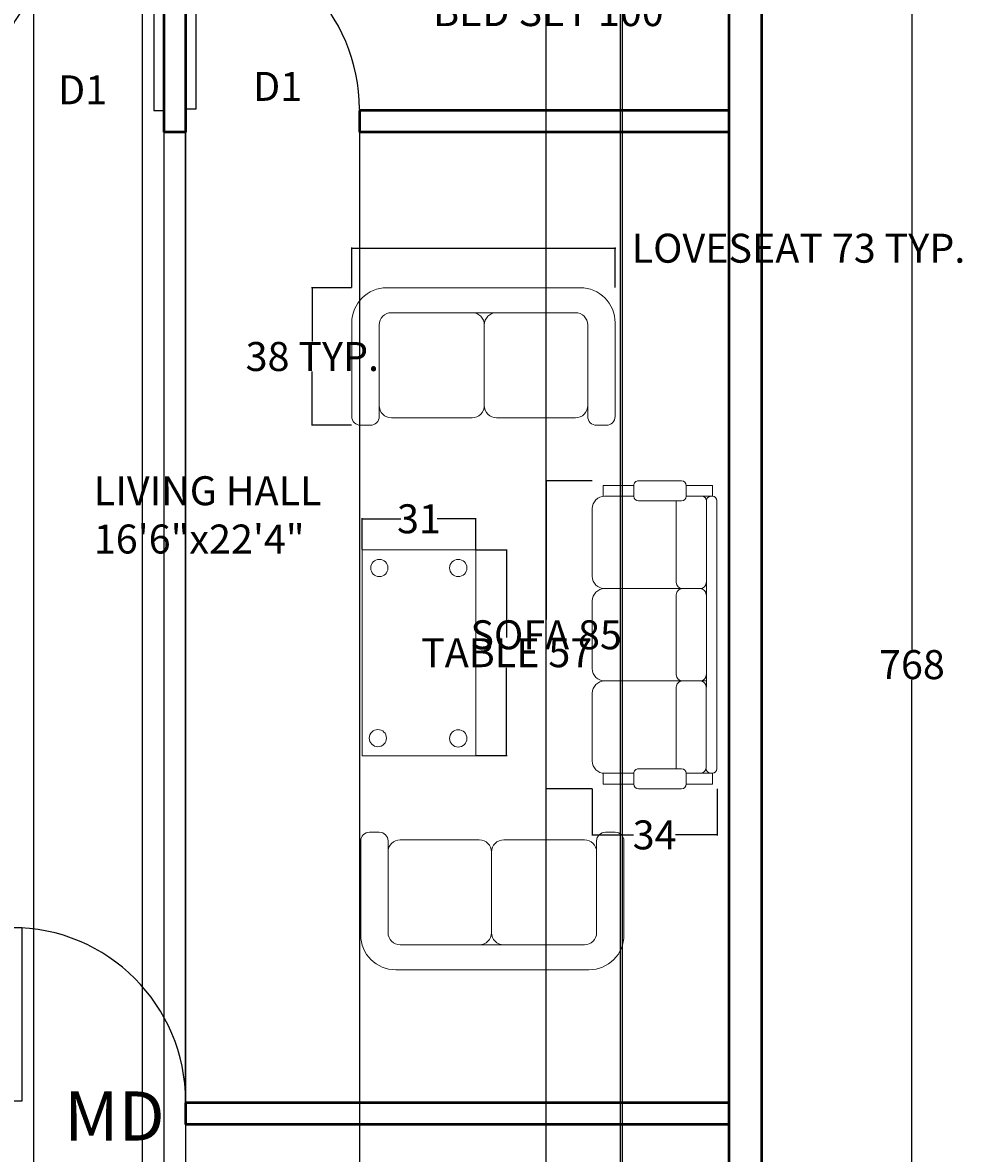
# Model space of a CAD drawing. Units: inches. Extents: x 3004 to 3478, y -798 to 114.
# Tile 4 of 5: x 3218 to 3478, y -503 to -190. Entities that reach past the tile are written whole.
import ezdxf

# ---------------------------------------------------------------- set-up
doc = ezdxf.new("R2010")
doc.units = ezdxf.units.IN
doc.header["$MEASUREMENT"] = 0
for name, color, linetype, lineweight in [('A-ANNO-DIMS', 2, 'Continuous', 18), ('A-ANNO-TEXT', 7, 'Continuous', 18), ('A-AREA-IDEN', 7, 'Continuous', 18), ('A-DOOR', 4, 'Continuous', 25), ('A-FURN', 8, 'Continuous', 18), ('A-WALL', 7, 'Continuous', 50)]:
    doc.layers.add(name, color=color, linetype=linetype, lineweight=lineweight)
doc.styles.get("Standard").update_dxf_attribs({"font": 'arial.ttf', "height": 8})
doc.dimstyles.get("Standard").update_dxf_attribs({"dimtxt": 0.18, "dimasz": 0.18, "dimexe": 0.18, "dimexo": 0.0625, "dimgap": 0.09, "dimtad": 0, "dimtih": 1, "dimtoh": 1, "dimzin": 0, "dimdsep": 46, "dimlunit": 4, "dimtxsty": 'Standard', "dimcen": 0.09, "dimadec": 0, "dimazin": 0, "dimtfac": 1, "dimtofl": 0, "dimtmove": 0, "dimatfit": 3, "dimfxl": 1, "dimtolj": 1, "dimtzin": 0, "dimarcsym": 0})

# ---------------------------------------------------------------- blocks, each defined once
blk = doc.blocks.new('F19')
for p, q in [((0.8306, 0.0191), (-0.9094, 0.0191)), ((-1.0094, -0.0109), (-0.9394, -0.0109)), ((-1.0094, -0.1809), (-1.0094, -0.0109)), ((-0.9394, -0.1809), (-0.9394, -0.0098)), ((-0.9394, -0.0109), (-0.9394, -0.0198)), ((0.213, -0.0498), (-0.9094, -0.0498)), ((-0.2985, -0.0498), (-0.387, -0.0498)), ((0.3015, -0.0498), (0.213, -0.0498)), ((0.2606, -0.6059), (0.2606, -0.0509)), ((0.3006, -0.0509), (0.8206, -0.0509)), ((0.9306, -0.0109), (0.8606, -0.0109)), ((0.8606, -0.0109), (0.8606, -0.0209)), ((0.8606, -0.0906), (0.8606, -0.0109)), ((0.9306, -0.1809), (0.9306, -0.0109)), ((-0.9394, -0.1773), (-0.9394, -0.0798)), ((-0.3394, -0.2054), (-0.3394, -0.0909)), ((0.2606, -0.2054), (0.2606, -0.0909)), ((0.8606, -0.1809), (0.8606, -0.0909)), ((-1.0394, -0.2109), (-1.0394, -0.4909)), ((-1.0094, -0.1809), (-0.9394, -0.1809)), ((-0.9094, -0.2109), (-0.9094, -0.4909)), ((-0.3394, -0.1546), (-0.3394, -0.6409)), ((0.2605, -0.3208), (0.2605, -0.174)), ((0.8306, -0.2109), (0.8306, -0.4909)), ((0.9306, -0.1809), (0.8606, -0.1809)), ((0.9606, -0.2109), (0.9606, -0.4909)), ((-0.3794, -0.2454), (-0.9114, -0.2454)), ((-0.3395, -0.3208), (-0.3395, -0.2854)), ((0.2206, -0.2454), (-0.2994, -0.2454)), ((0.2606, -0.2854), (0.2606, -0.6409)), ((0.829, -0.2454), (0.3006, -0.2454)), ((-1.0094, -0.5209), (-0.9394, -0.5209)), ((-1.0094, -0.7209), (-1.0094, -0.5209)), ((-0.9394, -0.5209), (-0.9394, -0.6909)), ((0.9306, -0.5209), (0.8606, -0.5209)), ((0.8606, -0.5209), (0.8606, -0.6909)), ((0.9306, -0.7209), (0.9306, -0.5209)), ((-0.9394, -0.6059), (-0.9394, -0.7109)), ((-0.9394, -0.6909), (-0.9394, -0.65)), ((-0.3394, -0.6059), (-0.3394, -0.7109)), ((0.2606, -0.6059), (0.2606, -0.7109)), ((0.8606, -0.6909), (0.8606, -0.65)), ((-0.9694, -0.7209), (-1.0094, -0.7209)), ((-0.9694, -0.7209), (-0.9393, -0.7209)), ((-0.9394, -0.6909), (-0.9394, -0.7109)), ((0.8906, -0.7209), (0.8605, -0.7209)), ((0.8606, -0.6909), (0.8606, -0.7109)), ((0.8906, -0.7209), (0.9306, -0.7209)), ((-0.4194, -0.7909), (-0.8594, -0.7909)), ((-0.4194, -0.7909), (-0.8594, -0.7909)), ((0.1806, -0.7909), (-0.2594, -0.7909)), ((0.0266, -0.7909), (0.0266, -0.7909)), ((0.7806, -0.7909), (0.3406, -0.7909))]:
    blk.add_line(p, q)
for centre, radius, start, end in [((-0.9094, -0.0109), 0.03, 90, 180), ((0.8306, -0.0109), 0.03, 360, 90), ((-0.9094, -0.0198), 0.03, 180, 270), ((-0.9094, -0.0798), 0.03, 90, 180), ((-0.3794, -0.0909), 0.04, 0, 90), ((-0.2994, -0.0909), 0.04, 90, 180), ((0.2206, -0.0909), 0.04, 0, 90), ((0.3006, -0.0909), 0.04, 90, 180), ((0.8206, -0.0909), 0.04, 0, 90), ((0.8306, -0.0209), 0.03, 270, 360), ((-1.0094, -0.2109), 0.03, 90, 180), ((-0.9394, -0.2109), 0.03, 0, 90), ((-0.3794, -0.2054), 0.04, 270, 360), ((-0.2994, -0.2054), 0.04, 180, 270), ((0.2206, -0.2054), 0.04, 270, 360), ((0.3006, -0.2054), 0.04, 180, 270), ((0.8606, -0.2109), 0.03, 90, 180), ((0.9306, -0.2109), 0.03, 0, 90), ((-1.0094, -0.4909), 0.03, 180, 270), ((-0.9394, -0.4909), 0.03, 270, 360), ((0.8606, -0.4909), 0.03, 180, 270), ((0.9306, -0.4909), 0.03, 270, 360), ((-0.8594, -0.7109), 0.08, 180, 270), ((-0.4194, -0.7109), 0.08, 270, 360), ((-0.4194, -0.7109), 0.08, 270, 360), ((-0.2594, -0.7109), 0.08, 180, 270), ((0.1806, -0.7109), 0.08, 270, 360), ((0.3406, -0.7109), 0.08, 180, 270), ((0.7806, -0.7109), 0.08, 270, 360)]:
    blk.add_arc(centre, radius, start, end)
blk = doc.blocks.new('A$C5C1B5EFD')
blk.add_blockref('F19', (1.0394, 0.7909))
blk = doc.blocks.new('A$C6BA70F2F')
for p, q in [((0.2, 0.7857), (1.3031, 0.7857)), ((0, 0.05), (0, 0.5857)), ((0.2263, 0.6431), (1.2768, 0.6431)), ((0.7563, 0.5835), (0.7563, 0.1071)), ((1.5031, 0.05), (1.5031, 0.5857)), ((0.1563, 0.05), (0.1563, 0.5731)), ((0.7563, 0.1131), (0.7563, 0.5731)), ((1.3468, 0.05), (1.3468, 0.5731)), ((0.6863, 0.0431), (0.2263, 0.0431)), ((1.2768, 0.0431), (0.8263, 0.0431)), ((0.1063, 0), (0.05, 0)), ((1.3968, 0), (1.4531, 0))]:
    blk.add_line(p, q)
for centre, radius, start, end in [((0.2, 0.5857), 0.2, 90, 180), ((1.3031, 0.5857), 0.2, 0, 90), ((0.2263, 0.5731), 0.07, 90, 180), ((0.6863, 0.5731), 0.07, 0, 90), ((0.8263, 0.5731), 0.07, 90, 180), ((1.2768, 0.5731), 0.07, 0, 90), ((0.2263, 0.1131), 0.07, 180, 270), ((0.6863, 0.1131), 0.07, 270, 0), ((0.8263, 0.1131), 0.07, 180, 270), ((1.2768, 0.1131), 0.07, 270, 0), ((0.05, 0.05), 0.05, 180, 270), ((0.1063, 0.05), 0.05, 270, 0), ((1.3968, 0.05), 0.05, 180, 270), ((1.4531, 0.05), 0.05, 270, 0)]:
    blk.add_arc(centre, radius, start, end)
blk = doc.blocks.new('table')
blk.add_lwpolyline([(-20.55, 0), (36.33, 0), (36.33, -31.34), (-20.55, -31.34)], close=True)
for centre in [(-15.51, -4.83), (31.56, -4.83), (-15.51, -26.62), (31.48, -27.03)]:
    blk.add_circle(centre, 2.38)
blk = doc.blocks.new('*U16')
for p, q in [((0, 0), (0, -100)), ((750, 0), (750, -100))]:
    blk.add_line(p, q)
blk.add_lwpolyline([(0, 0), (0, 750), (43.75, 750), (43.75, 0)], close=True)
blk.add_arc((0, 0), 750, 0, 90)
blk = doc.blocks.new('*U17')
for p, q in [((-750, 0), (-750, -100)), ((0, 0), (0, -100))]:
    blk.add_line(p, q)
blk.add_lwpolyline([(0, 0), (0, 750), (-43.75, 750), (-43.75, 0)], close=True)
blk.add_arc((0, 0), 750, 90, 180)
blk = doc.blocks.new('*D26')
at = {"layer": 'A-ANNO-DIMS', "color": 0, "lineweight": -2, "transparency": 16777216}
for p, q in [((3309.11, -263.53), (3309.11, -252.5)), ((3309.29, -252.68), (3381.63, -252.68)), ((3381.81, -263.53), (3381.81, -252.5)), ((3381.81, -252.68), (3381.99, -252.68))]:
    blk.add_line(p, q, dxfattribs=at)
at = {"layer": 'A-ANNO-DIMS', "color": 0, "transparency": 16777216}
for points in [[(3309.29, -252.65), (3309.29, -252.71), (3309.11, -252.68)], [(3381.63, -252.65), (3381.63, -252.71), (3381.81, -252.68)]]:
    blk.add_solid(points, dxfattribs=at)
at = {"layer": 'Defpoints', "color": 0, "transparency": 16777216}
for p in [(3381.81, -252.68), (3309.11, -263.59), (3381.81, -263.59)]:
    blk.add_point(p, dxfattribs=at)
at = {"layer": 'A-ANNO-DIMS', "color": 0, "transparency": 16777216, "insert": (3432.43, -252.68), "char_height": 8, "attachment_point": 5}
blk.add_mtext('\\A1;LOVESEAT 73 TYP.', dxfattribs=at)
blk = doc.blocks.new('*D27')
at = {"layer": 'A-ANNO-DIMS', "color": 0, "lineweight": -2, "transparency": 16777216}
for p, q in [((3309.04, -263.59), (3298.02, -263.59)), ((3298.2, -263.77), (3298.2, -278.41)), ((3298.2, -301.41), (3298.2, -286.77)), ((3309.04, -301.59), (3298.02, -301.59))]:
    blk.add_line(p, q, dxfattribs=at)
at = {"layer": 'A-ANNO-DIMS', "color": 0, "transparency": 16777216}
for points in [[(3298.17, -263.77), (3298.23, -263.77), (3298.2, -263.59)], [(3298.17, -301.41), (3298.23, -301.41), (3298.2, -301.59)]]:
    blk.add_solid(points, dxfattribs=at)
at = {"layer": 'Defpoints', "color": 0, "transparency": 16777216}
for p in [(3298.2, -263.59), (3309.11, -263.59), (3309.11, -301.59)]:
    blk.add_point(p, dxfattribs=at)
at = {"layer": 'A-ANNO-DIMS', "color": 0, "transparency": 16777216, "insert": (3298.2, -282.59), "char_height": 8, "attachment_point": 5}
blk.add_mtext('\\A1;38 TYP.', dxfattribs=at)
blk = doc.blocks.new('*D32')
at = {"layer": 'A-ANNO-DIMS', "color": 0, "lineweight": -2, "transparency": 16777216}
for p, q in [((3375.44, -316.93), (3362.58, -316.93)), ((3362.76, -317.11), (3362.76, -355.21)), ((3362.76, -401.77), (3362.76, -363.67)), ((3375.44, -401.95), (3362.58, -401.95))]:
    blk.add_line(p, q, dxfattribs=at)
at = {"layer": 'A-ANNO-DIMS', "color": 0, "transparency": 16777216}
for points in [[(3362.73, -317.11), (3362.79, -317.11), (3362.76, -316.93)], [(3362.73, -401.77), (3362.79, -401.77), (3362.76, -401.95)]]:
    blk.add_solid(points, dxfattribs=at)
at = {"layer": 'Defpoints', "color": 0, "transparency": 16777216}
for p in [(3375.51, -316.93), (3362.76, -401.95), (3375.51, -401.95)]:
    blk.add_point(p, dxfattribs=at)
at = {"layer": 'A-ANNO-DIMS', "color": 0, "transparency": 16777216, "insert": (3362.76, -359.44), "char_height": 8, "attachment_point": 5}
blk.add_mtext('\\A1;SOFA 85', dxfattribs=at)
blk = doc.blocks.new('*D33')
at = {"layer": 'A-ANNO-DIMS', "color": 0, "lineweight": -2, "transparency": 16777216}
for p, q in [((3375.51, -402.01), (3375.51, -414.88)), ((3409.94, -402.01), (3409.94, -414.88)), ((3375.69, -414.7), (3386.92, -414.7)), ((3409.76, -414.7), (3398.52, -414.7))]:
    blk.add_line(p, q, dxfattribs=at)
at = {"layer": 'A-ANNO-DIMS', "color": 0, "transparency": 16777216}
for points in [[(3375.69, -414.67), (3375.69, -414.73), (3375.51, -414.7)], [(3409.76, -414.67), (3409.76, -414.73), (3409.94, -414.7)]]:
    blk.add_solid(points, dxfattribs=at)
at = {"layer": 'Defpoints', "color": 0, "transparency": 16777216}
for p in [(3375.51, -401.95), (3409.94, -401.95), (3409.94, -414.7)]:
    blk.add_point(p, dxfattribs=at)
at = {"layer": 'A-ANNO-DIMS', "color": 0, "transparency": 16777216, "insert": (3392.72, -414.7), "char_height": 8, "attachment_point": 5}
blk.add_mtext('\\A1;34', dxfattribs=at)
blk = doc.blocks.new('*D34')
at = {"layer": 'A-ANNO-DIMS', "color": 0, "lineweight": -2, "transparency": 16777216}
for p, q in [((3313.57, -172.46), (3313.57, -187.52)), ((3413.21, -172.46), (3413.21, -187.52)), ((3313.75, -187.34), (3329.19, -187.34)), ((3413.03, -187.34), (3397.59, -187.34))]:
    blk.add_line(p, q, dxfattribs=at)
at = {"layer": 'A-ANNO-DIMS', "color": 0, "transparency": 16777216}
for points in [[(3313.75, -187.31), (3313.75, -187.37), (3313.57, -187.34)], [(3413.03, -187.31), (3413.03, -187.37), (3413.21, -187.34)]]:
    blk.add_solid(points, dxfattribs=at)
at = {"layer": 'Defpoints', "color": 0, "transparency": 16777216}
for p in [(3313.57, -172.39), (3413.21, -172.39), (3413.21, -187.34)]:
    blk.add_point(p, dxfattribs=at)
at = {"layer": 'A-ANNO-DIMS', "color": 0, "transparency": 16777216, "insert": (3363.39, -187.34), "char_height": 8, "attachment_point": 5}
blk.add_mtext('\\A1;BED SET 100', dxfattribs=at)
blk = doc.blocks.new('*D36')
at = {"layer": 'A-ANNO-DIMS', "color": 0, "lineweight": -2, "transparency": 16777216}
for p, q in [((3343.39, -335.95), (3352.04, -335.95)), ((3351.86, -336.13), (3351.86, -360.23)), ((3351.86, -392.64), (3351.86, -368.54)), ((3343.39, -392.82), (3352.04, -392.82))]:
    blk.add_line(p, q, dxfattribs=at)
at = {"layer": 'A-ANNO-DIMS', "color": 0, "transparency": 16777216}
for points in [[(3351.83, -336.13), (3351.89, -336.13), (3351.86, -335.95)], [(3351.83, -392.64), (3351.89, -392.64), (3351.86, -392.82)]]:
    blk.add_solid(points, dxfattribs=at)
at = {"layer": 'Defpoints', "color": 0, "transparency": 16777216}
for p in [(3343.33, -335.95), (3343.33, -392.82), (3351.86, -392.82)]:
    blk.add_point(p, dxfattribs=at)
at = {"layer": 'A-ANNO-DIMS', "color": 0, "transparency": 16777216, "insert": (3351.86, -364.39), "char_height": 8, "attachment_point": 5}
blk.add_mtext('\\A1;TABLE 57', dxfattribs=at)
blk = doc.blocks.new('*D37')
at = {"layer": 'A-ANNO-DIMS', "color": 0, "lineweight": -2, "transparency": 16777216}
for p, q in [((3311.98, -335.88), (3311.98, -327.23)), ((3312.16, -327.41), (3322.61, -327.41)), ((3343.15, -327.41), (3332.7, -327.41)), ((3343.33, -335.88), (3343.33, -327.23))]:
    blk.add_line(p, q, dxfattribs=at)
at = {"layer": 'A-ANNO-DIMS', "color": 0, "transparency": 16777216}
for points in [[(3312.16, -327.38), (3312.16, -327.44), (3311.98, -327.41)], [(3343.15, -327.38), (3343.15, -327.44), (3343.33, -327.41)]]:
    blk.add_solid(points, dxfattribs=at)
at = {"layer": 'Defpoints', "color": 0, "transparency": 16777216}
for p in [(3343.33, -327.41), (3311.98, -335.95), (3343.33, -335.95)]:
    blk.add_point(p, dxfattribs=at)
at = {"layer": 'A-ANNO-DIMS', "color": 0, "transparency": 16777216, "insert": (3327.65, -327.41), "char_height": 8, "attachment_point": 5}
blk.add_mtext('\\A1;31', dxfattribs=at)
blk = doc.blocks.new('*D39')
at = {"layer": 'A-ANNO-DIMS', "color": 0, "lineweight": -2, "transparency": 16777216}
for p, q in [((3422.27, 16.32), (3463.94, 16.32)), ((3463.76, 16.14), (3463.76, -363.5)), ((3463.76, -751.5), (3463.76, -371.85)), ((3422.27, -751.68), (3463.94, -751.68))]:
    blk.add_line(p, q, dxfattribs=at)
at = {"layer": 'A-ANNO-DIMS', "color": 0, "transparency": 16777216}
for points in [[(3463.73, 16.14), (3463.79, 16.14), (3463.76, 16.32)], [(3463.73, -751.5), (3463.79, -751.5), (3463.76, -751.68)]]:
    blk.add_solid(points, dxfattribs=at)
at = {"layer": 'Defpoints', "color": 0, "transparency": 16777216}
for p in [(3422.21, 16.32), (3422.21, -751.68), (3463.76, -751.68)]:
    blk.add_point(p, dxfattribs=at)
at = {"layer": 'A-ANNO-DIMS', "color": 0, "transparency": 16777216, "insert": (3463.76, -367.68), "char_height": 8, "attachment_point": 5}
blk.add_mtext('\\A1;768', dxfattribs=at)
blk = doc.blocks.new('*D44')
at = {"layer": 'A-ANNO-DIMS', "color": 0, "lineweight": -2, "transparency": 16777216}
for p, q in [((3257.211316, -220.74039), (3257.211316, -793.40789)), ((3263.211316, -220.74039), (3263.211316, -793.40789)), ((3257.031316, -793.22789), (3256.851316, -793.22789)), ((3263.391316, -793.22789), (3263.571316, -793.22789))]:
    blk.add_line(p, q, dxfattribs=at)
at = {"layer": 'A-ANNO-DIMS', "color": 0, "transparency": 16777216}
for points in [[(3257.031316, -793.19789), (3257.031316, -793.25789), (3257.211316, -793.22789)], [(3263.391316, -793.19789), (3263.391316, -793.25789), (3263.211316, -793.22789)]]:
    blk.add_solid(points, dxfattribs=at)
at = {"layer": 'Defpoints', "color": 0, "transparency": 16777216}
for p in [(3257.211316, -220.67789), (3263.211316, -220.67789), (3263.211316, -793.22789)]:
    blk.add_point(p, dxfattribs=at)
at = {"layer": 'A-ANNO-DIMS', "color": 0, "transparency": 16777216, "insert": (3260.211316, -793.22789), "char_height": 8, "attachment_point": 5}
blk.add_mtext('\\A1;6', dxfattribs=at)
blk = doc.blocks.new('*D45')
at = {"layer": 'A-ANNO-DIMS', "color": 0, "lineweight": -2, "transparency": 16777216}
for p, q in [((3422.21, 16.26), (3422.21, -793.41)), ((3413.21, 7.26), (3413.21, -793.41)), ((3413.39, -793.23), (3414.99, -793.23)), ((3422.03, -793.23), (3420.43, -793.23))]:
    blk.add_line(p, q, dxfattribs=at)
at = {"layer": 'A-ANNO-DIMS', "color": 0, "transparency": 16777216}
for points in [[(3413.39, -793.2), (3413.39, -793.26), (3413.21, -793.23)], [(3422.03, -793.2), (3422.03, -793.26), (3422.21, -793.23)]]:
    blk.add_solid(points, dxfattribs=at)
at = {"layer": 'Defpoints', "color": 0, "transparency": 16777216}
for p in [(3422.21, 16.32), (3413.21, 7.32), (3422.21, -793.23)]:
    blk.add_point(p, dxfattribs=at)
at = {"layer": 'A-ANNO-DIMS', "color": 0, "transparency": 16777216, "insert": (3417.71, -793.23), "char_height": 8, "attachment_point": 5}
blk.add_mtext('\\A1;9', dxfattribs=at)
blk = doc.blocks.new('*D46')
at = {"layer": 'A-ANNO-DIMS', "color": 0, "lineweight": -2, "transparency": 16777216}
for p, q in [((3263.21, -214.34), (3263.21, -793.41)), ((3311.21, -214.74), (3311.21, -793.41)), ((3263.39, -793.23), (3281.22, -793.23)), ((3311.03, -793.23), (3293.2, -793.23))]:
    blk.add_line(p, q, dxfattribs=at)
at = {"layer": 'A-ANNO-DIMS', "color": 0, "transparency": 16777216}
for points in [[(3263.39, -793.2), (3263.39, -793.26), (3263.21, -793.23)], [(3311.03, -793.2), (3311.03, -793.26), (3311.21, -793.23)]]:
    blk.add_solid(points, dxfattribs=at)
at = {"layer": 'Defpoints', "color": 0, "transparency": 16777216}
for p in [(3263.21, -214.28), (3311.21, -214.68), (3311.21, -793.23)]:
    blk.add_point(p, dxfattribs=at)
at = {"layer": 'A-ANNO-DIMS', "color": 0, "transparency": 16777216, "insert": (3287.21, -793.23), "char_height": 8, "attachment_point": 5}
blk.add_mtext('\\A1;48', dxfattribs=at)
blk = doc.blocks.new('*D47')
at = {"layer": 'A-ANNO-DIMS', "color": 0, "lineweight": -2, "transparency": 16777216}
for p, q in [((3413.21, -42.74), (3413.21, -793.41)), ((3383.21, -46.74), (3383.21, -793.41)), ((3383.39, -793.23), (3392.41, -793.23)), ((3413.03, -793.23), (3404.01, -793.23))]:
    blk.add_line(p, q, dxfattribs=at)
at = {"layer": 'A-ANNO-DIMS', "color": 0, "transparency": 16777216}
for points in [[(3383.39, -793.2), (3383.39, -793.26), (3383.21, -793.23)], [(3413.03, -793.2), (3413.03, -793.26), (3413.21, -793.23)]]:
    blk.add_solid(points, dxfattribs=at)
at = {"layer": 'Defpoints', "color": 0, "transparency": 16777216}
for p in [(3413.21, -42.68), (3383.21, -46.68), (3413.21, -793.23)]:
    blk.add_point(p, dxfattribs=at)
at = {"layer": 'A-ANNO-DIMS', "color": 0, "transparency": 16777216, "insert": (3398.21, -793.23), "char_height": 8, "attachment_point": 5}
blk.add_mtext('\\A1;30', dxfattribs=at)
blk = doc.blocks.new('*D55')
at = {"layer": 'A-ANNO-DIMS', "color": 0, "lineweight": -2, "transparency": 16777216}
for p, q in [((3215.21, -494.62), (3215.21, 109.05)), ((3215.39, 108.87), (3233.22, 108.87)), ((3263.03, 108.87), (3245.2, 108.87)), ((3263.21, -494.62), (3263.21, 109.05))]:
    blk.add_line(p, q, dxfattribs=at)
at = {"layer": 'A-ANNO-DIMS', "color": 0, "transparency": 16777216}
for points in [[(3215.39, 108.9), (3215.39, 108.84), (3215.21, 108.87)], [(3263.03, 108.9), (3263.03, 108.84), (3263.21, 108.87)]]:
    blk.add_solid(points, dxfattribs=at)
at = {"layer": 'Defpoints', "color": 0, "transparency": 16777216}
for p in [(3263.21, 108.87), (3215.21, -494.68), (3263.21, -494.68)]:
    blk.add_point(p, dxfattribs=at)
at = {"layer": 'A-ANNO-DIMS', "color": 0, "transparency": 16777216, "insert": (3239.21, 108.87), "char_height": 8, "attachment_point": 5}
blk.add_mtext('\\A1;48', dxfattribs=at)
blk = doc.blocks.new('*D59')
at = {"layer": 'A-ANNO-DIMS', "color": 0, "lineweight": -2, "transparency": 16777216}
for p, q in [((3362.72, -0.74), (3362.72, -793.41)), ((3383.72, -0.74), (3383.72, -793.41)), ((3362.9, -793.23), (3368.1, -793.23)), ((3383.54, -793.23), (3378.33, -793.23))]:
    blk.add_line(p, q, dxfattribs=at)
at = {"layer": 'A-ANNO-DIMS', "color": 0, "transparency": 16777216}
for points in [[(3362.9, -793.2), (3362.9, -793.26), (3362.72, -793.23)], [(3383.54, -793.2), (3383.54, -793.26), (3383.72, -793.23)]]:
    blk.add_solid(points, dxfattribs=at)
at = {"layer": 'Defpoints', "color": 0, "transparency": 16777216}
for p in [(3362.72, -0.68), (3383.72, -0.68), (3383.72, -793.23)]:
    blk.add_point(p, dxfattribs=at)
at = {"layer": 'A-ANNO-DIMS', "color": 0, "transparency": 16777216, "insert": (3373.22, -793.23), "char_height": 8, "attachment_point": 5}
blk.add_mtext('\\A1;21', dxfattribs=at)
blk = doc.blocks.new('*D63')
at = {"layer": 'A-ANNO-DIMS', "color": 0, "lineweight": -2, "transparency": 16777216}
for p, q in [((3221.21, -46.74), (3221.21, -793.41)), ((3251.21, -46.74), (3251.21, -793.41)), ((3221.39, -793.23), (3230.41, -793.23)), ((3251.03, -793.23), (3242.01, -793.23))]:
    blk.add_line(p, q, dxfattribs=at)
at = {"layer": 'A-ANNO-DIMS', "color": 0, "transparency": 16777216}
for points in [[(3221.39, -793.2), (3221.39, -793.26), (3221.21, -793.23)], [(3251.03, -793.2), (3251.03, -793.26), (3251.21, -793.23)]]:
    blk.add_solid(points, dxfattribs=at)
at = {"layer": 'Defpoints', "color": 0, "transparency": 16777216}
for p in [(3221.21, -46.68), (3251.21, -46.68), (3251.21, -793.23)]:
    blk.add_point(p, dxfattribs=at)
at = {"layer": 'A-ANNO-DIMS', "color": 0, "transparency": 16777216, "insert": (3236.21, -793.23), "char_height": 8, "attachment_point": 5}
blk.add_mtext('\\A1;30', dxfattribs=at)
blk = doc.blocks.new('*D64')
at = {"layer": 'A-ANNO-DIMS', "color": 0, "lineweight": -2, "transparency": 16777216}
for p, q in [((3215.21, -190.74), (3215.21, -793.41)), ((3257.21, -220.74), (3257.21, -793.41)), ((3215.39, -793.23), (3230.27, -793.23)), ((3257.03, -793.23), (3242.15, -793.23))]:
    blk.add_line(p, q, dxfattribs=at)
at = {"layer": 'A-ANNO-DIMS', "color": 0, "transparency": 16777216}
for points in [[(3215.39, -793.2), (3215.39, -793.26), (3215.21, -793.23)], [(3257.03, -793.2), (3257.03, -793.26), (3257.21, -793.23)]]:
    blk.add_solid(points, dxfattribs=at)
at = {"layer": 'Defpoints', "color": 0, "transparency": 16777216}
for p in [(3215.21, -190.68), (3257.21, -220.68), (3257.21, -793.23)]:
    blk.add_point(p, dxfattribs=at)
at = {"layer": 'A-ANNO-DIMS', "color": 0, "transparency": 16777216, "insert": (3236.21, -793.23), "char_height": 8, "attachment_point": 5}
blk.add_mtext('\\A1;42', dxfattribs=at)

msp = doc.modelspace()

# ---------------------------------------------------------------- linework, layer by layer
at = {"layer": 'A-WALL'}
for p, q in [((3422.2113, 16.3221), (3422.2113, -703.6779)), ((3413.2113, 7.3221), (3413.2113, -703.6779)), ((3263.2113, -40.6779), (3263.2113, -220.6779)), ((3257.2113, -46.6779), (3257.2113, -220.6779)), ((3413.2113, -214.6779), (3311.2113, -214.6779)), ((3311.2113, -214.6779), (3311.2113, -220.6779)), ((3263.2113, -220.6779), (3257.2113, -220.6779)), ((3413.2113, -220.6779), (3311.2113, -220.6779)), ((3413.2113, -488.6779), (3263.2113, -488.6779)), ((3263.2113, -488.6779), (3263.2113, -494.6779)), ((3413.2113, -494.6779), (3263.2113, -494.6779))]:
    msp.add_line(p, q, dxfattribs=at)

# ---------------------------------------------------------------- block references
at = {"layer": 'A-DOOR'}
for name, p, xscale, yscale, zscale in [('*U17', (3257.2113, -214.6779), 0.0639999999999998, 0.0639999999999998, 0.0639999999999998), ('*U16', (3263.2113, -214.2779), 0.0639999999999998, 0.0639999999999998, 0.0639999999999998), ('*U16', (3215.2113, -488.2779), 0.0640000000000003, 0.0640000000000003, 0.0640000000000003)]:
    msp.add_blockref(name, p, dxfattribs=dict(at, xscale=xscale, yscale=yscale, zscale=zscale))
at = {"layer": 'A-FURN', "xscale": 48.36981152459372, "yscale": 48.36981152459372, "zscale": 48.36981152459372}
msp.add_blockref('A$C6BA70F2F', (3309.1052, -301.591), dxfattribs=at)
at = {"layer": 'A-FURN'}
for name, p, xscale, yscale, zscale, rotation in [('A$C5C1B5EFD', (3375.507, -316.9327), 42.50631032504036, 42.50631032504036, 42.50631032504036, 270), ('A$C6BA70F2F', (3384.2585, -413.963), 48.36981152459372, 48.36981152459372, 48.36981152459372, 180)]:
    msp.add_blockref(name, p, dxfattribs=dict(at, xscale=xscale, yscale=yscale, zscale=zscale, rotation=rotation))
at = {"layer": 'A-FURN', "rotation": 270}
msp.add_blockref('table', (3343.3251, -356.4975), dxfattribs=at)

# ---------------------------------------------------------------- texts
at = {"layer": 'A-ANNO-TEXT', "attachment_point": 1}
for s, width, gutter_width, insert, char_height in [('D1', 22.083935, 40, (3227.9906, -204.9434), 8), ('D1', 22.083935, 40, (3281.8389, -203.9911), 8), ('MD', 37.429582, 67.7951, (3229.6849, -485.5599), 13.55903)]:
    msp.add_mtext_dynamic_manual_height_columns(s, width=width, gutter_width=gutter_width, heights=[0], dxfattribs=dict(at, insert=insert, char_height=char_height))
at = {"layer": 'A-AREA-IDEN', "insert": (3237.8699, -315.659), "char_height": 8, "attachment_point": 1}
msp.add_mtext_dynamic_manual_height_columns('LIVING HALL\\P16\'6"x22\'4"', width=228.23715, gutter_width=40, heights=[0], dxfattribs=at)

# ---------------------------------------------------------------- dimensions: what is measured, and where the dimension line sits
at = {"layer": 'A-ANNO-DIMS'}
for base, p1, p2, picture, middle in [((3263.2113, 108.8721), (3215.2113, -494.6779), (3263.2113, -494.6779), '*D55', (3239.2113, 108.8721)), ((3422.2113, -793.2279), (3413.2113, 7.3221), (3422.2113, 16.3221), '*D45', (3417.7113, -793.2279)), ((3383.7177, -793.2279), (3362.7177, -0.6779), (3383.7177, -0.6779), '*D59', (3373.2177, -793.2279)), ((3413.2113, -793.2279), (3383.2113, -46.6779), (3413.2113, -42.6779), '*D47', (3398.2113, -793.2279)), ((3251.2113, -793.2279), (3221.2113, -46.6779), (3251.2113, -46.6779), '*D63', (3236.2113, -793.2279)), ((3257.2113, -793.2279), (3215.2113, -190.6779), (3257.2113, -220.6779), '*D64', (3236.2113, -793.2279)), ((3311.2113, -793.2279), (3263.2113, -214.2779), (3311.2113, -214.6779), '*D46', (3287.2113, -793.2279)), ((3263.2113, -793.2279), (3257.2113, -220.6779), (3263.2113, -220.6779), '*D44', (3260.2113, -793.2279)), ((3343.3251, -327.4148), (3311.9843, -335.9465), (3343.3251, -335.9465), '*D37', (3327.6547, -327.4148)), ((3409.9371, -414.6972), (3375.507, -401.9453), (3409.9371, -401.9453), '*D33', (3392.7221, -414.6972))]:
    dim = msp.add_linear_dim(base=base, p1=p1, p2=p2, dimstyle='Standard', override={"dimdec": 0, "dimlfac": 1, "dimrnd": 0, "dimzin": 0, "dimdsep": 46, "dimlunit": 2}, dxfattribs=at)
    dim.commit()
    dim.dimension.update_dxf_attribs({"geometry": picture, "text_midpoint": middle})
dim = msp.add_linear_dim(base=(3463.7613, -751.6779), p1=(3422.2113, 16.3221), p2=(3422.2113, -751.6779), angle=90, dimstyle='Standard', override={"dimdec": 0, "dimlfac": 1, "dimrnd": 0, "dimzin": 0, "dimdsep": 46, "dimlunit": 2}, dxfattribs=at)
dim.commit()
dim.dimension.update_dxf_attribs({"geometry": '*D39', "text_midpoint": (3463.7613, -367.6779)})
for base, p1, p2, text, picture, middle in [((3413.2113, -187.3399), (3313.5676, -172.3933), (3413.2113, -172.3933), 'BED SET <>', '*D34', (3363.3895, -187.3399)), ((3381.8101, -252.6834), (3309.1052, -263.5892), (3381.8101, -263.5892), 'LOVESEAT <> TYP.', '*D26', (3432.4293, -252.6834))]:
    dim = msp.add_linear_dim(base=base, p1=p1, p2=p2, text=text, dimstyle='Standard', override={"dimdec": 0, "dimlfac": 1, "dimrnd": 0, "dimzin": 0, "dimdsep": 46, "dimlunit": 2}, dxfattribs=at)
    dim.commit()
    dim.dimension.update_dxf_attribs({"geometry": picture, "text_midpoint": middle})
for base, p1, p2, angle, text, picture, middle in [((3298.1995, -263.5892), (3309.1052, -301.591), (3309.1052, -263.5892), 90, '<> TYP.', '*D27', (3298.1995, -282.5901)), ((3362.7551, -401.9453), (3375.507, -316.9327), (3375.507, -401.9453), 270, 'SOFA <>', '*D32', (3362.7551, -359.439)), ((3351.8568, -392.8246), (3343.3251, -335.9465), (3343.3251, -392.8246), 270, 'TABLE <>', '*D36', (3351.8568, -364.3855))]:
    dim = msp.add_linear_dim(base=base, p1=p1, p2=p2, angle=angle, text=text, dimstyle='Standard', override={"dimdec": 0, "dimlfac": 1, "dimrnd": 0, "dimzin": 0, "dimdsep": 46, "dimlunit": 2}, dxfattribs=at)
    dim.commit()
    dim.dimension.update_dxf_attribs({"geometry": picture, "text_midpoint": middle})

doc.saveas('drawing.dxf')
